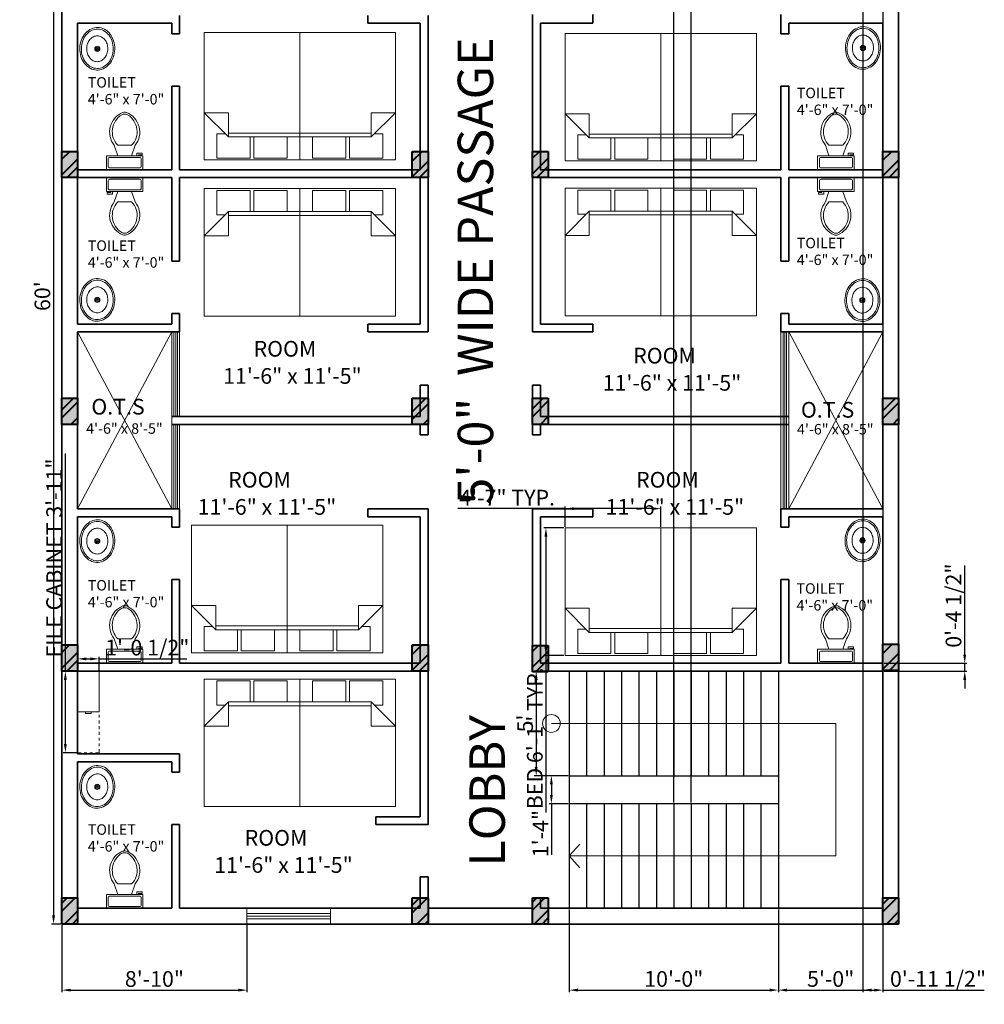
# Model space of a CAD drawing. Units: inches. Extents: x 2507 to 5802, y 1229 to 3238.
# Tile 1 of 2: x 2532 to 3085, y 1229 to 1794. Entities that reach past the tile are written whole.
import ezdxf

# ---------------------------------------------------------------- set-up
doc = ezdxf.new("R2010")
doc.units = ezdxf.units.IN
for name, color, linetype, lineweight, true_color in [('A-ANNO-DIMS', 244, 'Continuous', 18, 0x991b1e), ('A-AREA-IDEN', 146, 'Continuous', 18, 0x105689), ('A-FLOR-FIXT', 244, 'Continuous', 18, 0x991b1e), ('A-FLOR-OPEN', 244, 'Continuous', 13, 0x991b1e), ('A-FURN', 146, 'Continuous', 18, 0x105689), ('A-GLAZ', 146, 'Continuous', 18, 0x105689)]:
    doc.layers.add(name, color=color, linetype=linetype, lineweight=lineweight, true_color=true_color)
for name, color, linetype, lineweight in [('A-ANNO-SYMB', 7, 'Continuous', 18), ('A-COLS', 7, 'Continuous', 40), ('A-FLOR-STRS', 7, 'Continuous', 25), ('A-WALL', 7, 'Continuous', 35)]:
    doc.layers.add(name, color=color, linetype=linetype, lineweight=lineweight)
doc.styles.get("Standard").update_dxf_attribs({"font": 'arial.ttf'})
doc.dimstyles.new('ISO-25', dxfattribs={"dimtxt": 9, "dimasz": 5, "dimexe": 1.25, "dimexo": 0.625, "dimtad": 1, "dimdec": 0, "dimlunit": 3, "dimtxsty": 'Standard', "dimcen": 2.5, "dimadec": 0, "dimazin": 0, "dimtfac": 1, "dimtdec": 0, "dimtmove": 0, "dimatfit": 3, "dimfxl": 1, "dimarcsym": 0})
pattern_1 = [(45, (-3102.79, -1462.177), (-6.735192, 6.735192), []), (45, (-3098.3, -1462.177), (-6.735192, 6.735192), [])]

# ---------------------------------------------------------------- blocks, each defined once
blk = doc.blocks.new('Bed - Queen')
for p, q in [((0, -80.00003), (0, 0)), ((0, 0), (59.99999, 0)), ((59.99999, 0), (59.99999, -80.00003)), ((7.99999, -1.2), (28.79998, -1.2)), ((7.99999, -14.4), (7.99999, -1.2)), ((28.79998, -1.2), (28.79998, -14.4)), ((31.19999, -1.2), (51.99999, -1.2)), ((31.19999, -14.4), (31.19999, -1.2)), ((51.99999, -1.2), (51.99999, -16.4)), ((0, -14.4), (44.8, -14.4)), ((44.8, -16.8), (0, -16.8)), ((59.99999, -29.6), (44.8, -14.4)), ((44.8, -14.4), (44.8, -29.6)), ((51.99999, -16.4), (46.79936, -16.4)), ((44.8, -29.6), (59.99999, -29.6)), ((59.99999, -80.00003), (0, -80.00003))]:
    blk.add_line(p, q)
blk = doc.blocks.new('*D3')
at = {"layer": 'A-ANNO-DIMS', "color": 0, "lineweight": -2, "transparency": 16777216}
for p, q in [((2555.37, 1995.09), (2549.93, 1995.09)), ((2551.18, 1990.09), (2551.18, 1280.09)), ((2555.37, 1275.09), (2549.93, 1275.09))]:
    blk.add_line(p, q, dxfattribs=at)
at = {"layer": 'A-ANNO-DIMS', "color": 0, "transparency": 16777216}
for points in [[(2550.35, 1990.09), (2552.02, 1990.09), (2551.18, 1995.09)], [(2550.35, 1280.09), (2552.02, 1280.09), (2551.18, 1275.09)]]:
    blk.add_solid(points, dxfattribs=at)
at = {"layer": 'Defpoints', "color": 0, "transparency": 16777216}
for p in [(2555.99, 1995.09), (2551.18, 1275.09), (2555.99, 1275.09)]:
    blk.add_point(p, dxfattribs=at)
at = {"layer": 'A-ANNO-DIMS', "color": 0, "transparency": 16777216, "insert": (2545.96, 1635.09), "char_height": 9, "attachment_point": 5, "rotation": 90}
blk.add_mtext("60'", dxfattribs=at)
blk = doc.blocks.new('Toilet - top')
for p, q in [((9.5, -6), (9.5, -2)), ((-10, -8.5), (-8, -8.5)), ((-10, -9.5), (-10, -8.5)), ((-7, -9.5), (-10, -9.5)), ((-8, -8.5), (-8, -8)), ((-7, -8), (-7, -9.5)), ((-4, -8), (-6, -14)), ((4, -8), (6, -14)), ((4, -14), (-4, -14))]:
    blk.add_line(p, q)
blk.add_lwpolyline([(10.5, -8), (10.5, 0), (-10.5, 0), (-10.5, -8)], close=True)
for points in [[(-9.5, -2), (-9.5, -6)], [(8.5, -1), (-8.5, -1)], [(-8.5, -7), (8.5, -7)]]:
    blk.add_lwpolyline(points)
for centre, radius, start, end in [((-8.62, -1.88), 0.884, 81.8699, 188.1301), ((8.62, -1.88), 0.884, 351.8699, 98.1301), ((-8.62, -6.12), 0.884, 171.8699, 278.1301), ((8.62, -6.12), 0.884, 261.8699, 8.1301), ((3.52, -21.58), 12.17, 141.4691, 247.9714), ((4.2, -21.82), 11.33, 136.3677, 238.9468), ((-3.52, -21.58), 12.17, 292.0284, 38.5307), ((-4.2, -21.82), 11.33, 301.053, 43.6321), ((0, -27.88), 4, 245.7318, 294.2682), ((0, -29), 4, 254.8605, 285.1395)]:
    blk.add_arc(centre, radius, start, end)
blk = doc.blocks.new('Sink - Oval top')
for p, q in [((-1, 0), (1, 0)), ((0, 1), (0, -1))]:
    blk.add_line(p, q)
for points in [[(-12.23, 0.39, 0.117634), (-11.46, -3.36, 0.104469), (-8.88, -6.8, 0.090016), (-5.08, -9.07, 0.08192), (-0.32, -10.02, 0.08192), (4.49, -9.38, 0.090016), (8.42, -7.36, 0.104469), (11.22, -4.09, 0.117634), (12.23, -0.39, 0.117634), (11.46, 3.36, 0.104469), (8.88, 6.8, 0.090016), (5.08, 9.07, 0.08192), (0.32, 10.02, 0.08192), (-4.49, 9.38, 0.090016), (-8.42, 7.36, 0.104469), (-11.22, 4.09, 0.117634)], [(-11.29, 0.16, 0.118622), (-10.52, -3.25, 0.104678), (-8.07, -6.36, 0.089562), (-4.54, -8.37, 0.081185), (-0.13, -9.15, 0.081185), (4.3, -8.49, 0.089562), (7.89, -6.58, 0.104678), (10.42, -3.55, 0.118622), (11.29, -0.16, 0.118622), (10.52, 3.25, 0.104678), (8.07, 6.36, 0.089562), (4.54, 8.37, 0.081185), (0.13, 9.15, 0.081185), (-4.3, 8.49, 0.089562), (-7.89, 6.58, 0.104678), (-10.42, 3.55, 0.118622)], [(-7.42, 0.08, 0.118283), (-6.91, -2.17, 0.104607), (-5.29, -4.21, 0.089718), (-2.97, -5.53, 0.081436), (-0.07, -6.04, 0.081436), (2.84, -5.59, 0.089718), (5.2, -4.33, 0.104607), (6.86, -2.32, 0.118283), (7.42, -0.08, 0.118283), (6.91, 2.17, 0.104607), (5.29, 4.21, 0.089718), (2.97, 5.53, 0.081436), (0.07, 6.04, 0.081436), (-2.84, 5.59, 0.089718), (-5.2, 4.33, 0.104607), (-6.86, 2.32, 0.118283)]]:
    blk.add_lwpolyline(points, format="xyb", close=True)
for radius in [1.5, 1]:
    blk.add_circle((0, 0), radius)
blk = doc.blocks.new('File Cabinet - Letter')
for p, q in [((0, 0), (15, 0)), ((0, -28.5), (0, 0)), ((15, 0), (15, -28.5)), ((15, -28.5), (0, -28.5)), ((0, -29.5), (0, -28.5)), ((0, -33.5), (0, -31.5)), ((5.5, -28.5), (5.5, -29.5)), ((5.5, -29.5), (9.5, -29.5)), ((9.5, -29.5), (9.5, -28.5)), ((15, -30.5), (15, -32.5)), ((0, -37.5), (0, -35.5)), ((0, -41.5), (0, -39.5)), ((15, -34.5), (15, -36.5)), ((15, -38.5), (15, -40.5)), ((0, -45.5), (0, -43.5)), ((0, -49.5), (0, -47.5)), ((15, -42.5), (15, -44.5)), ((15, -46.5), (15, -48.5)), ((0, -53.5), (0, -51.5)), ((15, -50.5), (15, -52.5)), ((15, -54.5), (15, -57)), ((0, -57), (0, -55.5)), ((2.5, -57), (0, -57)), ((6.5, -57), (4.5, -57)), ((10.5, -57), (8.5, -57)), ((15, -57), (12.5, -57))]:
    blk.add_line(p, q)
blk = doc.blocks.new('*D8')
at = {"layer": 'A-ANNO-DIMS', "color": 0, "lineweight": -2, "transparency": 16777216}
for p, q in [((2846.37, 1420.09), (2826.8, 1420.09)), ((2828.05, 1415.09), (2828.05, 1365.09)), ((2846.37, 1360.09), (2826.8, 1360.09))]:
    blk.add_line(p, q, dxfattribs=at)
at = {"layer": 'A-ANNO-DIMS', "color": 0, "transparency": 16777216}
for points in [[(2827.21, 1415.09), (2828.88, 1415.09), (2828.05, 1420.09)], [(2827.21, 1365.09), (2828.88, 1365.09), (2828.05, 1360.09)]]:
    blk.add_solid(points, dxfattribs=at)
at = {"layer": 'Defpoints', "color": 0, "transparency": 16777216}
for p in [(2846.99, 1420.09), (2828.05, 1360.09), (2846.99, 1360.09)]:
    blk.add_point(p, dxfattribs=at)
at = {"layer": 'A-ANNO-DIMS', "color": 0, "transparency": 16777216, "insert": (2822.85, 1390.09), "char_height": 9, "attachment_point": 5, "rotation": 90}
blk.add_mtext("5'", dxfattribs=at)
blk = doc.blocks.new('*D9')
at = {"layer": 'A-ANNO-DIMS', "color": 0, "lineweight": -2, "transparency": 16777216}
for p, q in [((2846.37, 1360.09), (2835.52, 1360.09)), ((2836.77, 1355.09), (2836.77, 1349.09)), ((2846.37, 1344.09), (2835.52, 1344.09)), ((2836.77, 1344.09), (2836.77, 1314.76))]:
    blk.add_line(p, q, dxfattribs=at)
at = {"layer": 'A-ANNO-DIMS', "color": 0, "transparency": 16777216}
for points in [[(2835.93, 1355.09), (2837.6, 1355.09), (2836.77, 1360.09)], [(2835.93, 1349.09), (2837.6, 1349.09), (2836.77, 1344.09)]]:
    blk.add_solid(points, dxfattribs=at)
at = {"layer": 'Defpoints', "color": 0, "transparency": 16777216}
for p in [(2846.99, 1360.09), (2836.77, 1344.09), (2846.99, 1344.09)]:
    blk.add_point(p, dxfattribs=at)
at = {"layer": 'A-ANNO-DIMS', "color": 0, "transparency": 16777216, "insert": (2831.62, 1326.93), "char_height": 9, "attachment_point": 5, "rotation": 90}
blk.add_mtext('1\'-4"', dxfattribs=at)
blk = doc.blocks.new('COL-9x15')
h = blk.add_hatch()
h.set_pattern_fill('ANSI32', color=256)
h.set_pattern_definition(pattern_1)
h.paths.add_polyline_path([(9, 15), (0, 15), (0, 0), (9, 0)])
h = blk.add_hatch()
h.set_pattern_fill('ANSI32', color=256)
h.set_pattern_definition(pattern_1)
h.paths.add_polyline_path([(9, 15), (0, 15), (0, 0), (9, 0)])
at = {"transparency": 33554687}
h = blk.add_hatch(dxfattribs=at)
h.set_pattern_fill('ANSI32', color=256)
h.set_pattern_definition(pattern_1)
h.paths.add_polyline_path([(9, 15), (0, 15), (0, 0), (9, 0)])
h = blk.add_hatch(color=256, dxfattribs=at)
h.dxf.hatch_style = 1
h.paths.add_polyline_path([(9, 15), (0, 15), (0, 0), (9, 0)])
for p, q in [((0, 15), (9, 15)), ((0, 0), (0, 15)), ((9, 15), (9, 0)), ((9, 0), (0, 0))]:
    blk.add_line(p, q)
blk = doc.blocks.new('WIN-48x9')
for p, q in [((0, 9), (48, 9)), ((0, 0), (0, 9)), ((0, 6), (48, 6)), ((48, 9), (48, 0)), ((0, 4.5), (48, 4.5)), ((0, 3), (48, 3)), ((48, 0), (0, 0))]:
    blk.add_line(p, q)
blk = doc.blocks.new('OTS-OPENING-MARK-54x101_5')
for p, q in [((0, 101.5), (54, 0)), ((0, 0), (54, 101.5))]:
    blk.add_line(p, q)
blk = doc.blocks.new('*D15')
at = {"layer": 'A-ANNO-DIMS', "color": 0, "lineweight": -2, "transparency": 16777216}
for p, q in [((2843.99, 1502.28), (2832.39, 1502.28)), ((2833.64, 1497.28), (2833.64, 1434.11)), ((2843.99, 1429.11), (2832.39, 1429.11)), ((2833.64, 1429.11), (2833.64, 1339.06))]:
    blk.add_line(p, q, dxfattribs=at)
at = {"layer": 'A-ANNO-DIMS', "color": 0, "transparency": 16777216}
for points in [[(2832.8, 1497.28), (2834.47, 1497.28), (2833.64, 1502.28)], [(2832.8, 1434.11), (2834.47, 1434.11), (2833.64, 1429.11)]]:
    blk.add_solid(points, dxfattribs=at)
at = {"layer": 'Defpoints', "color": 0, "transparency": 16777216}
for p in [(2844.61, 1502.28), (2833.64, 1429.11), (2844.61, 1429.11)]:
    blk.add_point(p, dxfattribs=at)
at = {"layer": 'A-ANNO-DIMS', "color": 0, "transparency": 16777216, "insert": (2828.42, 1381.58), "char_height": 9, "attachment_point": 5, "rotation": 90}
blk.add_mtext('BED 6\'-1" TYP.', dxfattribs=at)
blk = doc.blocks.new('*D16')
at = {"layer": 'A-ANNO-DIMS', "color": 0, "lineweight": -2, "transparency": 16777216}
for p, q in [((2844.61, 1513.26), (2783.14, 1513.26)), ((2844.61, 1502.91), (2844.61, 1514.51)), ((2894.49, 1513.26), (2849.61, 1513.26)), ((2899.49, 1502.91), (2899.49, 1514.51))]:
    blk.add_line(p, q, dxfattribs=at)
at = {"layer": 'A-ANNO-DIMS', "color": 0, "transparency": 16777216}
for points in [[(2849.61, 1514.09), (2849.61, 1512.43), (2844.61, 1513.26)], [(2894.49, 1514.09), (2894.49, 1512.43), (2899.49, 1513.26)]]:
    blk.add_solid(points, dxfattribs=at)
at = {"layer": 'Defpoints', "color": 0, "transparency": 16777216}
for p in [(2844.61, 1513.26), (2844.61, 1502.28), (2899.49, 1502.28)]:
    blk.add_point(p, dxfattribs=at)
at = {"layer": 'A-ANNO-DIMS', "color": 0, "transparency": 16777216, "insert": (2811.38, 1518.39), "char_height": 9, "attachment_point": 5}
blk.add_mtext('4\'-7" TYP.', dxfattribs=at)
blk = doc.blocks.new('*D23')
at = {"layer": 'A-ANNO-DIMS', "color": 0, "lineweight": -2, "transparency": 16777216}
for p, q in [((2557.97, 1420.09), (2557.97, 1544.78)), ((2564.37, 1420.09), (2556.72, 1420.09)), ((2557.97, 1378.29), (2557.97, 1415.09)), ((2564.37, 1373.29), (2556.72, 1373.29))]:
    blk.add_line(p, q, dxfattribs=at)
at = {"layer": 'A-ANNO-DIMS', "color": 0, "transparency": 16777216}
for points in [[(2557.14, 1415.09), (2558.8, 1415.09), (2557.97, 1420.09)], [(2557.14, 1378.29), (2558.8, 1378.29), (2557.97, 1373.29)]]:
    blk.add_solid(points, dxfattribs=at)
at = {"layer": 'Defpoints', "color": 0, "transparency": 16777216}
for p in [(2557.97, 1420.09), (2564.99, 1420.09), (2564.99, 1373.29)]:
    blk.add_point(p, dxfattribs=at)
at = {"layer": 'A-ANNO-DIMS', "color": 0, "transparency": 16777216, "insert": (2552.69, 1484.93), "char_height": 9, "attachment_point": 5, "rotation": 90}
blk.add_mtext('FILE CABINET 3\'-11"', dxfattribs=at)
blk = doc.blocks.new('*D24')
at = {"layer": 'A-ANNO-DIMS', "color": 0, "lineweight": -2, "transparency": 16777216}
for p, q in [((2564.99, 1420.72), (2564.99, 1428.36)), ((2577.31, 1420.72), (2577.31, 1428.36)), ((2569.99, 1427.11), (2572.31, 1427.11)), ((2577.31, 1427.11), (2627.6, 1427.11))]:
    blk.add_line(p, q, dxfattribs=at)
at = {"layer": 'A-ANNO-DIMS', "color": 0, "transparency": 16777216}
for points in [[(2569.99, 1427.94), (2569.99, 1426.28), (2564.99, 1427.11)], [(2572.31, 1427.94), (2572.31, 1426.28), (2577.31, 1427.11)]]:
    blk.add_solid(points, dxfattribs=at)
at = {"layer": 'Defpoints', "color": 0, "transparency": 16777216}
for p in [(2577.31, 1427.11), (2564.99, 1420.09), (2577.31, 1420.09)]:
    blk.add_point(p, dxfattribs=at)
at = {"layer": 'A-ANNO-DIMS', "color": 0, "transparency": 16777216, "insert": (2604.96, 1432.39), "char_height": 9, "attachment_point": 5}
blk.add_mtext('1\'-0 1/2"', dxfattribs=at)
blk = doc.blocks.new('*D27')
at = {"layer": 'A-ANNO-DIMS', "color": 0, "lineweight": -2, "transparency": 16777216}
for p, q in [((2555.99, 1274.47), (2555.99, 1235.94)), ((2662.12, 1274.47), (2662.12, 1235.94)), ((2560.99, 1237.19), (2657.12, 1237.19))]:
    blk.add_line(p, q, dxfattribs=at)
at = {"layer": 'A-ANNO-DIMS', "color": 0, "transparency": 16777216}
for points in [[(2560.99, 1238.02), (2560.99, 1236.36), (2555.99, 1237.19)], [(2657.12, 1238.02), (2657.12, 1236.36), (2662.12, 1237.19)]]:
    blk.add_solid(points, dxfattribs=at)
at = {"layer": 'Defpoints', "color": 0, "transparency": 16777216}
for p in [(2555.99, 1275.09), (2662.12, 1275.09), (2662.12, 1237.19)]:
    blk.add_point(p, dxfattribs=at)
at = {"layer": 'A-ANNO-DIMS', "color": 0, "transparency": 16777216, "insert": (2609.06, 1242.41), "char_height": 9, "attachment_point": 5}
blk.add_mtext('8\'-10"', dxfattribs=at)
blk = doc.blocks.new('*D28')
at = {"layer": 'A-ANNO-DIMS', "color": 0, "lineweight": -2, "transparency": 16777216}
for p, q in [((2846.99, 1283.47), (2846.99, 1235.94)), ((2966.99, 1283.47), (2966.99, 1235.94)), ((2851.99, 1237.19), (2961.99, 1237.19))]:
    blk.add_line(p, q, dxfattribs=at)
at = {"layer": 'A-ANNO-DIMS', "color": 0, "transparency": 16777216}
for points in [[(2851.99, 1238.02), (2851.99, 1236.36), (2846.99, 1237.19)], [(2961.99, 1238.02), (2961.99, 1236.36), (2966.99, 1237.19)]]:
    blk.add_solid(points, dxfattribs=at)
at = {"layer": 'Defpoints', "color": 0, "transparency": 16777216}
for p in [(2846.99, 1284.09), (2966.99, 1284.09), (2966.99, 1237.19)]:
    blk.add_point(p, dxfattribs=at)
at = {"layer": 'A-ANNO-DIMS', "color": 0, "transparency": 16777216, "insert": (2906.99, 1242.41), "char_height": 9, "attachment_point": 5}
blk.add_mtext('10\'-0"', dxfattribs=at)
blk = doc.blocks.new('*D29')
at = {"layer": 'A-ANNO-DIMS', "color": 0, "lineweight": -2, "transparency": 16777216}
for p, q in [((2966.99, 1283.47), (2966.99, 1235.94)), ((3026.99, 1283.47), (3026.99, 1235.94)), ((2971.99, 1237.19), (3021.99, 1237.19))]:
    blk.add_line(p, q, dxfattribs=at)
at = {"layer": 'A-ANNO-DIMS', "color": 0, "transparency": 16777216}
for points in [[(2971.99, 1238.02), (2971.99, 1236.36), (2966.99, 1237.19)], [(3021.99, 1238.02), (3021.99, 1236.36), (3026.99, 1237.19)]]:
    blk.add_solid(points, dxfattribs=at)
at = {"layer": 'Defpoints', "color": 0, "transparency": 16777216}
for p in [(2966.99, 1284.09), (3026.99, 1284.09), (3026.99, 1237.19)]:
    blk.add_point(p, dxfattribs=at)
at = {"layer": 'A-ANNO-DIMS', "color": 0, "transparency": 16777216, "insert": (2996.99, 1242.41), "char_height": 9, "attachment_point": 5}
blk.add_mtext('5\'-0"', dxfattribs=at)
blk = doc.blocks.new('*D34')
at = {"layer": 'A-ANNO-DIMS', "color": 0, "lineweight": -2, "transparency": 16777216}
for p, q in [((2901.99, 2032.99), (2896.99, 2032.99)), ((2906.99, 1344.72), (2906.99, 2034.24)), ((2906.99, 2032.99), (2916.99, 2032.99)), ((2916.99, 1344.72), (2916.99, 2034.24)), ((2921.99, 2032.99), (2959.16, 2032.99))]:
    blk.add_line(p, q, dxfattribs=at)
at = {"layer": 'A-ANNO-DIMS', "color": 0, "transparency": 16777216}
for points in [[(2901.99, 2033.82), (2901.99, 2032.16), (2906.99, 2032.99)], [(2921.99, 2033.82), (2921.99, 2032.16), (2916.99, 2032.99)]]:
    blk.add_solid(points, dxfattribs=at)
at = {"layer": 'Defpoints', "color": 0, "transparency": 16777216}
for p in [(2916.99, 2032.99), (2906.99, 1344.09), (2916.99, 1344.09)]:
    blk.add_point(p, dxfattribs=at)
at = {"layer": 'A-ANNO-DIMS', "color": 0, "transparency": 16777216, "insert": (2943.07, 2038.21), "char_height": 9, "attachment_point": 5}
blk.add_mtext('0\'-10"', dxfattribs=at)
blk = doc.blocks.new('*D35')
at = {"layer": 'A-ANNO-DIMS', "color": 0, "lineweight": -2, "transparency": 16777216}
for p, q in [((3073.89, 1429.59), (3073.89, 1480.74)), ((3027.62, 1424.59), (3075.14, 1424.59)), ((3073.89, 1420.09), (3073.89, 1424.59)), ((3027.62, 1420.09), (3075.14, 1420.09)), ((3073.89, 1415.09), (3073.89, 1410.09))]:
    blk.add_line(p, q, dxfattribs=at)
at = {"layer": 'A-ANNO-DIMS', "color": 0, "transparency": 16777216}
for points in [[(3073.06, 1429.59), (3074.72, 1429.59), (3073.89, 1424.59)], [(3073.06, 1415.09), (3074.72, 1415.09), (3073.89, 1420.09)]]:
    blk.add_solid(points, dxfattribs=at)
at = {"layer": 'Defpoints', "color": 0, "transparency": 16777216}
for p in [(3026.99, 1424.59), (3073.89, 1424.59), (3026.99, 1420.09)]:
    blk.add_point(p, dxfattribs=at)
at = {"layer": 'A-ANNO-DIMS', "color": 0, "transparency": 16777216, "insert": (3068.61, 1457.66), "char_height": 9, "attachment_point": 5, "rotation": 90}
blk.add_mtext('0\'-4 1/2"', dxfattribs=at)
blk = doc.blocks.new('*D37')
at = {"layer": 'A-ANNO-DIMS', "color": 0, "lineweight": -2, "transparency": 16777216}
for p, q in [((3015.43, 1914.46), (3015.43, 1235.94)), ((3026.99, 1901.47), (3026.99, 1235.94)), ((3020.43, 1237.19), (3021.99, 1237.19)), ((3026.99, 1237.19), (3085.13, 1237.19))]:
    blk.add_line(p, q, dxfattribs=at)
at = {"layer": 'A-ANNO-DIMS', "color": 0, "transparency": 16777216}
for points in [[(3020.43, 1238.02), (3020.43, 1236.36), (3015.43, 1237.19)], [(3021.99, 1238.02), (3021.99, 1236.36), (3026.99, 1237.19)]]:
    blk.add_solid(points, dxfattribs=at)
at = {"layer": 'Defpoints', "color": 0, "transparency": 16777216}
for p in [(3015.43, 1915.08), (3026.99, 1902.09), (3026.99, 1237.19)]:
    blk.add_point(p, dxfattribs=at)
at = {"layer": 'A-ANNO-DIMS', "color": 0, "transparency": 16777216, "insert": (3058.56, 1242.47), "char_height": 9, "attachment_point": 5}
blk.add_mtext('0\'-11 1/2"', dxfattribs=at)

msp = doc.modelspace()

# ---------------------------------------------------------------- linework, layer by layer
at = {"layer": 'A-ANNO-SYMB'}
for p, q in [((2846.99, 1390.09), (2836.78, 1390.09)), ((2846.99, 1390.09), (2966.99, 1390.09)), ((2966.99, 1390.09), (2999.99, 1390.09)), ((2999.99, 1390.09), (2999.99, 1314.09)), ((2846.99, 1314.09), (2853.13, 1320.88)), ((2999.99, 1314.09), (2846.99, 1314.09)), ((2846.99, 1314.09), (2853.13, 1307.31))]:
    msp.add_line(p, q, dxfattribs=at)
msp.add_circle((2836.78, 1390.09), 5.1, dxfattribs=at)
at = {"layer": 'A-FLOR-STRS'}
for p, q in [((2846.99, 1420.09), (2846.99, 1344.09)), ((2856.99, 1420.09), (2856.99, 1360.09)), ((2866.99, 1420.09), (2866.99, 1360.09)), ((2876.99, 1420.09), (2876.99, 1360.09)), ((2886.99, 1420.09), (2886.99, 1360.09)), ((2896.99, 1420.09), (2896.99, 1360.09)), ((2906.99, 1420.09), (2906.99, 1360.09)), ((2916.99, 1420.09), (2916.99, 1360.09)), ((2926.99, 1420.09), (2926.99, 1360.09)), ((2936.99, 1420.09), (2936.99, 1360.09)), ((2946.99, 1420.09), (2946.99, 1360.09)), ((2956.99, 1420.09), (2956.99, 1360.09)), ((2966.99, 1420.09), (2966.99, 1344.09)), ((2846.99, 1360.09), (2966.99, 1360.09)), ((2966.99, 1344.09), (2846.99, 1344.09)), ((2846.99, 1344.09), (2846.99, 1284.09)), ((2856.99, 1344.09), (2856.99, 1284.09)), ((2866.99, 1344.09), (2866.99, 1284.09)), ((2876.99, 1344.09), (2876.99, 1284.09)), ((2886.99, 1344.09), (2886.99, 1284.09)), ((2896.99, 1344.09), (2896.99, 1284.09)), ((2906.99, 1344.09), (2906.99, 1284.09)), ((2916.99, 1344.09), (2916.99, 1284.09)), ((2926.99, 1344.09), (2926.99, 1284.09)), ((2936.99, 1344.09), (2936.99, 1284.09)), ((2946.99, 1344.09), (2946.99, 1284.09)), ((2956.99, 1344.09), (2956.99, 1284.09)), ((2966.99, 1344.09), (2966.99, 1284.09))]:
    msp.add_line(p, q, dxfattribs=at)
at = {"layer": 'A-GLAZ'}
for p, q in [((2618.99, 1614.59), (2618.99, 1513.09)), ((2623.49, 1614.59), (2618.99, 1614.59)), ((2620.24, 1614.59), (2620.24, 1566.09)), ((2621.24, 1614.59), (2621.24, 1566.09)), ((2622.24, 1614.59), (2622.24, 1566.09)), ((2623.49, 1614.59), (2623.49, 1566.09)), ((2968.49, 1614.59), (2968.49, 1513.09)), ((2968.49, 1614.59), (2972.99, 1614.59)), ((2969.74, 1614.59), (2969.74, 1513.09)), ((2970.74, 1614.59), (2970.74, 1513.09)), ((2971.74, 1614.59), (2971.74, 1513.09)), ((2972.99, 1614.59), (2972.99, 1513.09)), ((2620.24, 1561.59), (2620.24, 1513.09)), ((2621.24, 1561.59), (2621.24, 1513.09)), ((2622.24, 1561.59), (2622.24, 1513.09)), ((2623.49, 1561.59), (2623.49, 1513.09))]:
    msp.add_line(p, q, dxfattribs=at)
at = {"layer": 'A-WALL'}
for p, q in [((2555.99, 1275.09), (2555.99, 1995.09)), ((3035.99, 1995.09), (3035.99, 1275.09)), ((2623.49, 1785.59), (2623.49, 1796.09)), ((2731.49, 1791.59), (2731.49, 1796.09)), ((2765.99, 1755.59), (2765.99, 1796.09)), ((2825.99, 1755.59), (2825.99, 1796.59)), ((2860.49, 1791.59), (2860.49, 1796.59)), ((2968.49, 1785.59), (2968.49, 1796.59)), ((2564.99, 1791.59), (2618.99, 1791.59)), ((2564.99, 1707.59), (2564.99, 1791.59)), ((2618.99, 1785.59), (2618.99, 1791.59)), ((2731.49, 1791.59), (2761.49, 1791.59)), ((2761.49, 1755.59), (2761.49, 1791.59)), ((2830.49, 1755.59), (2830.49, 1791.59)), ((2830.49, 1791.59), (2860.49, 1791.59)), ((2972.99, 1791.59), (3026.99, 1791.59)), ((2972.99, 1785.59), (2972.99, 1791.59)), ((3026.99, 1791.59), (3026.99, 1707.59)), ((2618.99, 1785.59), (2623.49, 1785.59)), ((2968.49, 1785.59), (2972.99, 1785.59)), ((2968.49, 1785.59), (2972.99, 1785.59)), ((2618.99, 1755.59), (2623.49, 1755.59)), ((2618.99, 1707.59), (2618.99, 1755.59)), ((2623.49, 1707.59), (2623.49, 1755.59)), ((2761.49, 1707.59), (2761.49, 1755.59)), ((2765.99, 1614.59), (2765.99, 1755.59)), ((2825.99, 1614.59), (2825.99, 1755.59)), ((2830.49, 1707.59), (2830.49, 1755.59)), ((2968.49, 1755.59), (2972.99, 1755.59)), ((2968.49, 1755.59), (2972.99, 1755.59)), ((2968.49, 1707.59), (2968.49, 1755.59)), ((2972.99, 1707.59), (2972.99, 1755.59)), ((2564.99, 1707.59), (2618.99, 1707.59)), ((2623.49, 1707.59), (2761.49, 1707.59)), ((2830.49, 1707.59), (2968.49, 1707.59)), ((2972.99, 1707.59), (3026.99, 1707.59)), ((2564.99, 1703.09), (2618.99, 1703.09)), ((2564.99, 1619.09), (2564.99, 1703.09)), ((2618.99, 1655.09), (2618.99, 1703.09)), ((2623.49, 1655.09), (2623.49, 1703.09)), ((2623.49, 1703.09), (2761.49, 1703.09)), ((2761.49, 1619.09), (2761.49, 1703.09)), ((2830.49, 1703.09), (2968.49, 1703.09)), ((2830.49, 1619.09), (2830.49, 1703.09)), ((2968.49, 1655.09), (2968.49, 1703.09)), ((2972.99, 1655.09), (2972.99, 1703.09)), ((2972.99, 1703.09), (3026.99, 1703.09)), ((3026.99, 1703.09), (3026.99, 1619.09)), ((2618.99, 1655.09), (2623.49, 1655.09)), ((2968.49, 1655.09), (2972.99, 1655.09)), ((2618.99, 1625.09), (2623.49, 1625.09)), ((2618.99, 1619.09), (2618.99, 1625.09)), ((2623.49, 1614.59), (2623.49, 1625.09)), ((2968.49, 1625.09), (2972.99, 1625.09)), ((2968.49, 1614.59), (2968.49, 1625.09)), ((2972.99, 1619.09), (2972.99, 1625.09)), ((2564.99, 1619.09), (2618.99, 1619.09)), ((2731.49, 1619.09), (2761.49, 1619.09)), ((2731.49, 1614.59), (2731.49, 1619.09)), ((2830.49, 1619.09), (2860.49, 1619.09)), ((2860.49, 1614.59), (2860.49, 1619.09)), ((2972.99, 1619.09), (3026.99, 1619.09)), ((2564.99, 1614.59), (2623.49, 1614.59)), ((2564.99, 1566.09), (2564.99, 1614.59)), ((2731.49, 1614.59), (2765.99, 1614.59)), ((2825.99, 1614.59), (2860.49, 1614.59)), ((2968.49, 1614.59), (3026.99, 1614.59)), ((3026.99, 1614.59), (3026.99, 1513.09)), ((2761.49, 1584.09), (2765.99, 1584.09)), ((2761.49, 1566.09), (2761.49, 1584.09)), ((2765.99, 1555.59), (2765.99, 1584.09)), ((2825.99, 1584.09), (2830.49, 1584.09)), ((2825.99, 1555.59), (2825.99, 1584.09)), ((2830.49, 1566.09), (2830.49, 1584.09)), ((2618.99, 1566.09), (2761.49, 1566.09)), ((2830.49, 1566.09), (2972.99, 1566.09)), ((2564.99, 1513.09), (2564.99, 1561.59)), ((2618.99, 1561.59), (2761.49, 1561.59)), ((2761.49, 1555.59), (2761.49, 1561.59)), ((2830.49, 1561.59), (2972.99, 1561.59)), ((2830.49, 1555.59), (2830.49, 1561.59)), ((2761.49, 1555.59), (2765.99, 1555.59)), ((2825.99, 1555.59), (2830.49, 1555.59)), ((2564.99, 1513.09), (2623.49, 1513.09)), ((2623.49, 1502.59), (2623.49, 1513.09)), ((2731.49, 1508.59), (2731.49, 1513.09)), ((2731.49, 1513.09), (2765.99, 1513.09)), ((2731.49, 1508.59), (2731.49, 1513.09)), ((2765.99, 1332.09), (2765.99, 1513.09)), ((2825.99, 1513.09), (2860.49, 1513.09)), ((2825.99, 1419.76), (2825.99, 1513.09)), ((2860.49, 1508.59), (2860.49, 1513.09)), ((2968.49, 1502.59), (2968.49, 1513.09)), ((2968.49, 1513.09), (3026.99, 1513.09)), ((2564.99, 1508.59), (2618.99, 1508.59)), ((2564.99, 1424.59), (2564.99, 1508.59)), ((2618.99, 1502.59), (2618.99, 1508.59)), ((2731.49, 1508.59), (2761.49, 1508.59)), ((2761.49, 1424.59), (2761.49, 1508.59)), ((2830.49, 1508.59), (2860.49, 1508.59)), ((2830.49, 1424.59), (2830.49, 1508.59)), ((2972.99, 1502.59), (2972.99, 1508.59)), ((2972.99, 1508.59), (3026.99, 1508.59)), ((3026.99, 1508.59), (3026.99, 1424.59)), ((2618.99, 1502.59), (2623.49, 1502.59)), ((2968.49, 1502.59), (2972.99, 1502.59)), ((2618.99, 1472.59), (2623.49, 1472.59)), ((2618.99, 1424.59), (2618.99, 1472.59)), ((2623.49, 1424.59), (2623.49, 1472.59)), ((2968.49, 1424.59), (2968.49, 1472.59)), ((2968.49, 1472.59), (2972.99, 1472.59)), ((2972.99, 1424.59), (2972.99, 1472.59)), ((2564.99, 1424.59), (2618.99, 1424.59)), ((2623.49, 1424.59), (2761.49, 1424.59)), ((2830.49, 1424.59), (2968.49, 1424.59)), ((2972.99, 1424.59), (3026.99, 1424.59)), ((2564.99, 1420.09), (2761.49, 1420.09)), ((2564.99, 1372.59), (2564.99, 1420.09)), ((2761.49, 1336.59), (2761.49, 1420.09)), ((2830.49, 1420.09), (3026.99, 1420.09)), ((2830.49, 1419.76), (2830.49, 1420.09)), ((3026.99, 1420.09), (3026.99, 1284.09)), ((2623.49, 1372.59), (2564.99, 1372.59)), ((2623.49, 1362.09), (2623.49, 1372.59)), ((2564.99, 1284.09), (2564.99, 1368.09)), ((2618.99, 1368.09), (2564.99, 1368.09)), ((2618.99, 1362.09), (2618.99, 1368.09)), ((2623.49, 1362.09), (2618.99, 1362.09)), ((2761.49, 1336.59), (2735.99, 1336.59)), ((2735.99, 1336.59), (2735.99, 1332.09)), ((2618.99, 1284.09), (2618.99, 1332.09)), ((2623.49, 1332.09), (2618.99, 1332.09)), ((2623.49, 1284.09), (2623.49, 1332.09)), ((2765.99, 1332.09), (2735.99, 1332.09)), ((2765.99, 1332.09), (2761.49, 1332.09)), ((2761.49, 1284.09), (2761.49, 1302.09)), ((2765.99, 1302.09), (2761.49, 1302.09)), ((2765.99, 1284.09), (2765.99, 1302.09)), ((2825.99, 1284.09), (2825.99, 1290.09)), ((2830.49, 1284.09), (2830.49, 1290.09)), ((2618.99, 1284.09), (2564.99, 1284.09)), ((2761.49, 1284.09), (2623.49, 1284.09)), ((2825.99, 1284.09), (2765.99, 1284.09)), ((3026.99, 1284.09), (2830.49, 1284.09)), ((3035.99, 1275.09), (2555.99, 1275.09))]:
    msp.add_line(p, q, dxfattribs=at)

# ---------------------------------------------------------------- block references
at = {"layer": 'A-COLS'}
for p in [(2555.99, 1703.09), (2756.99, 1703.09), (2825.99, 1703.09), (3026.99, 1703.09), (2555.99, 1561.59), (2756.99, 1561.59), (2825.99, 1561.59), (3026.99, 1561.59), (2555.99, 1420.09), (2756.99, 1420.09), (2825.99, 1419.76), (3026.99, 1420.47), (2555.99, 1275.09), (2756.99, 1275.09), (2825.99, 1275.09), (3026.99, 1275.09)]:
    msp.add_blockref('COL-9x15', p, dxfattribs=at)
at = {"layer": 'A-FLOR-FIXT'}
for name, p, rotation in [('Sink - Oval top', (2576.27, 1776.95), 90), ('Sink - Oval top', (3015.5, 1777.39), 90), ('Toilet - top', (2591.99, 1707.59), 180), ('Toilet - top', (2999.99, 1707.59), 180), ('Sink - Oval top', (2576.27, 1632.97), 90), ('Sink - Oval top', (3015.17, 1632.8), 90), ('Sink - Oval top', (2576.27, 1494.65), 90), ('Sink - Oval top', (3015.29, 1495.06), 90), ('Toilet - top', (2591.99, 1424.59), 180), ('Toilet - top', (2999.99, 1424.59), 180), ('Sink - Oval top', (2576.27, 1353.73), 90), ('Toilet - top', (2591.99, 1284.09), 180)]:
    msp.add_blockref(name, p, dxfattribs=dict(at, rotation=rotation))
for p in [(2591.99, 1703.09), (2999.99, 1703.09)]:
    msp.add_blockref('Toilet - top', p, dxfattribs=at)
at = {"layer": 'A-FLOR-OPEN'}
for p in [(2564.99, 1513.09), (2972.99, 1513.09)]:
    msp.add_blockref('OTS-OPENING-MARK-54x101_5', p, dxfattribs=at)
at = {"layer": 'A-FURN', "yscale": 0.9146343891503859, "zscale": 0.9146343891503859, "rotation": 180}
for p, xscale in [((2692.49, 1713.19), 0.9146343891503859), ((2692.49, 1713.19), -0.9146343891503859), ((2899.49, 1712.62), 0.9146343891503859), ((2899.49, 1712.62), -0.9146343891503859), ((2685.17, 1430.63), 0.9146343891503859), ((2685.17, 1430.63), -0.9146343891503859), ((2899.49, 1429.11), 0.9146343891503859), ((2899.49, 1429.11), -0.9146343891503859)]:
    msp.add_blockref('Bed - Queen', p, dxfattribs=dict(at, xscale=xscale))
at = {"layer": 'A-FURN'}
for name, p, xscale, yscale, zscale in [('Bed - Queen', (2692.49, 1696.76), -0.9146343891503859, 0.9146343891503859, 0.9146343891503859), ('Bed - Queen', (2692.49, 1696.76), 0.9146343891503859, 0.9146343891503859, 0.9146343891503859), ('Bed - Queen', (2899.49, 1697.03), -0.9146343891503859, 0.9146343891503859, 0.9146343891503859), ('Bed - Queen', (2899.49, 1697.03), 0.9146343891503859, 0.9146343891503859, 0.9146343891503859), ('File Cabinet - Letter', (2564.99, 1420.09), 0.8210602793899477, 0.8210602793899477, 0.8210602793899477), ('Bed - Queen', (2692.49, 1415.56), -0.9146343891503859, 0.9146343891503859, 0.9146343891503859), ('Bed - Queen', (2692.49, 1415.56), 0.9146343891503859, 0.9146343891503859, 0.9146343891503859)]:
    msp.add_blockref(name, p, dxfattribs=dict(at, xscale=xscale, yscale=yscale, zscale=zscale))
at = {"layer": 'A-GLAZ'}
msp.add_blockref('WIN-48x9', (2662.12, 1275.09), dxfattribs=at)

# ---------------------------------------------------------------- texts
at = {"layer": 'A-AREA-IDEN'}
for s, height, p in [('5\'-0"  WIDE PASSAGE', 20.3499, (2803.37, 1515.56)), ('LOBBY ', 20.35, (2810.11, 1308.02))]:
    msp.add_text(s, height=height, rotation=90, dxfattribs=at).set_placement(p)
for s, height, p in [('TOILET', 6, (2570.81, 1754.67)), ('4\'-6" x 7\'-0"', 6, (2570.81, 1745.03)), ('TOILET', 6, (2977.56, 1748.59)), ('4\'-6" x 7\'-0"', 6, (2977.56, 1738.95)), ('TOILET', 6, (2570.81, 1661.07)), ('TOILET', 6, (2977.56, 1662.56)), ('4\'-6" x 7\'-0"', 6, (2570.81, 1651.43)), ('4\'-6" x 7\'-0"', 6, (2977.56, 1652.92)), ('ROOM', 9, (2665.93, 1600.42)), ('ROOM', 9, (2883.69, 1596.48)), ('11\'-6" x 11\'-5"', 9, (2648.46, 1584.84)), ('11\'-6" x 11\'-5"', 9, (2866.22, 1580.89)), ('O.T.S', 9, (2572.87, 1567.22)), ('O.T.S', 9, (2979.92, 1565.43)), ('4\'-6" x 8\'-5"', 6, (2569.89, 1556.2)), ('4\'-6" x 8\'-5"', 6, (2977.68, 1555.79)), ('ROOM', 9, (2651.33, 1525.33)), ('ROOM', 9, (2885.35, 1525.33)), ('11\'-6" x 11\'-5"', 9, (2633.86, 1509.75)), ('11\'-6" x 11\'-5"', 9, (2867.88, 1509.75)), ('TOILET', 6, (2570.81, 1466.3)), ('TOILET', 6, (2977.41, 1464.46)), ('4\'-6" x 7\'-0"', 6, (2570.81, 1456.67)), ('4\'-6" x 7\'-0"', 6, (2977.41, 1454.83)), ('TOILET', 6, (2570.81, 1326.25)), ('ROOM', 9, (2660.82, 1320.01)), ('4\'-6" x 7\'-0"', 6, (2570.81, 1316.62)), ('11\'-6" x 11\'-5"', 9, (2643.35, 1304.43))]:
    msp.add_text(s, height=height, dxfattribs=at).set_placement(p)

# ---------------------------------------------------------------- dimensions: what is measured, and where the dimension line sits
at = {"layer": 'A-ANNO-DIMS'}
for base, p1, p2, picture, middle in [((2916.99, 2032.99), (2906.99, 1344.09), (2916.99, 1344.09), '*D34', (2943.07, 2038.21)), ((3026.99, 1237.19), (3015.43, 1915.08), (3026.99, 1902.09), '*D37', (3058.56, 1242.47)), ((2577.31, 1427.11), (2564.99, 1420.09), (2577.31, 1420.09), '*D24', (2604.96, 1432.39)), ((2966.99, 1237.19), (2846.99, 1284.09), (2966.99, 1284.09), '*D28', (2906.99, 1242.41)), ((3026.99, 1237.19), (2966.99, 1284.09), (3026.99, 1284.09), '*D29', (2996.99, 1242.41)), ((2662.12, 1237.19), (2555.99, 1275.09), (2662.12, 1275.09), '*D27', (2609.06, 1242.41))]:
    dim = msp.add_linear_dim(base=base, p1=p1, p2=p2, dimstyle='ISO-25', override={"dimdec": 1, "dimlfac": 1, "dimrnd": 0, "dimzin": 1, "dimdsep": 46, "dimlunit": 4, "dimfrac": 2}, dxfattribs=at)
    dim.commit()
    dim.dimension.update_dxf_attribs({"geometry": picture, "text_midpoint": middle})
for base, p1, p2, override, picture, middle in [((2551.18, 1275.09), (2555.99, 1995.09), (2555.99, 1275.09), {"dimclrd": 0, "dimclre": 0, "dimclrt": 0}, '*D3', (2545.96, 1635.09)), ((3073.89, 1424.59), (3026.99, 1420.09), (3026.99, 1424.59), {"dimdec": 1, "dimlfac": 1, "dimrnd": 0, "dimzin": 1, "dimdsep": 46, "dimlunit": 4, "dimfrac": 2}, '*D35', (3068.61, 1457.66)), ((2828.05, 1360.09), (2846.99, 1420.09), (2846.99, 1360.09), {"dimclrd": 0, "dimclre": 0, "dimclrt": 0}, '*D8', (2822.85, 1390.09)), ((2836.77, 1344.09), (2846.99, 1360.09), (2846.99, 1344.09), {"dimclrd": 0, "dimclre": 0, "dimclrt": 0}, '*D9', (2831.62, 1326.93))]:
    dim = msp.add_linear_dim(base=base, p1=p1, p2=p2, angle=90, dimstyle='ISO-25', override=override, dxfattribs=at)
    dim.commit()
    dim.dimension.update_dxf_attribs({"geometry": picture, "text_midpoint": middle})
for base, p1, p2, angle, text, picture, middle in [((2557.97, 1420.09), (2564.99, 1373.29), (2564.99, 1420.09), 90, 'FILE CABINET <>', '*D23', (2552.69, 1484.93)), ((2844.61, 1513.26), (2899.49, 1502.28), (2844.61, 1502.28), 180, '<> TYP.', '*D16', (2811.38, 1518.39)), ((2833.64, 1429.11), (2844.61, 1502.28), (2844.61, 1429.11), 270, 'BED <> TYP.', '*D15', (2828.42, 1381.58))]:
    dim = msp.add_linear_dim(base=base, p1=p1, p2=p2, angle=angle, text=text, dimstyle='ISO-25', override={"dimdec": 1, "dimlfac": 1, "dimrnd": 0, "dimzin": 1, "dimdsep": 46, "dimlunit": 4, "dimfrac": 2}, dxfattribs=at)
    dim.commit()
    dim.dimension.update_dxf_attribs({"geometry": picture, "text_midpoint": middle})

doc.saveas('drawing.dxf')
